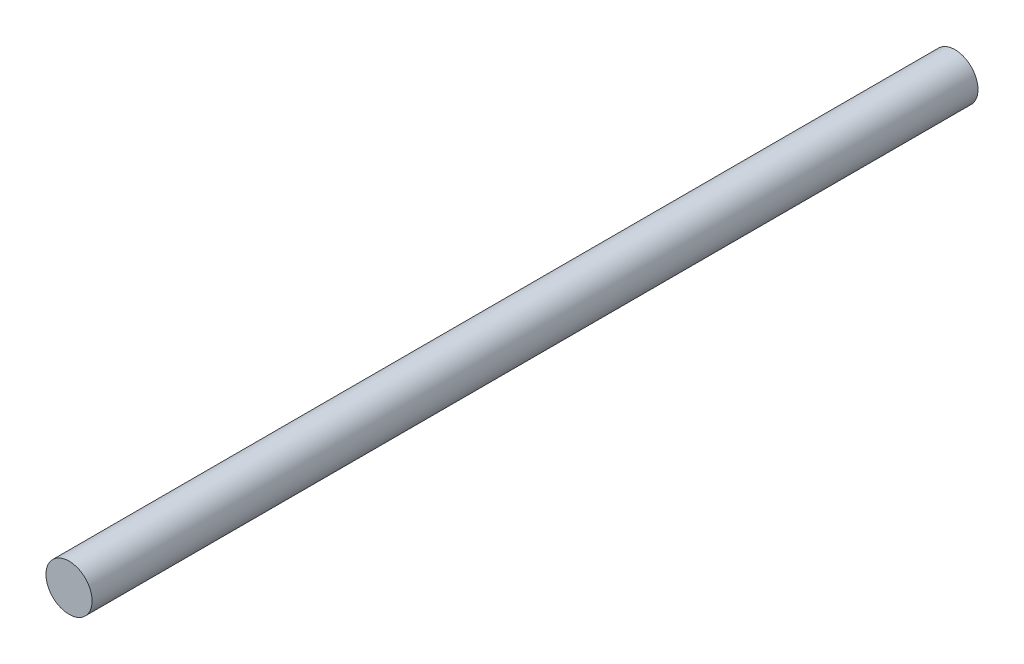
SolidWorks part; units mm, degrees
material "Plain Carbon Steel"
ref_plane "Front Plane" through (0, 0, 0) normal (0, 0, 1) x (1, 0, 0)
ref_plane "Top Plane" through (0, 0, 0) normal (0, 1, 0) x (1, 0, 0)
ref_plane "Right Plane" through (0, 0, 0) normal (1, 0, 0) x (0, 0, -1)
sketch "Rod Profile Ø5" plane through (0, 0, 0) normal (0, 0, 1) x (1, 0, 0)
  circle A0 centre (0, 0) radius 2.5
  dimension "D1" = 5
extrude "Rod Ø5x96" add sketch "Rod Profile Ø5" along normal mid plane 96
